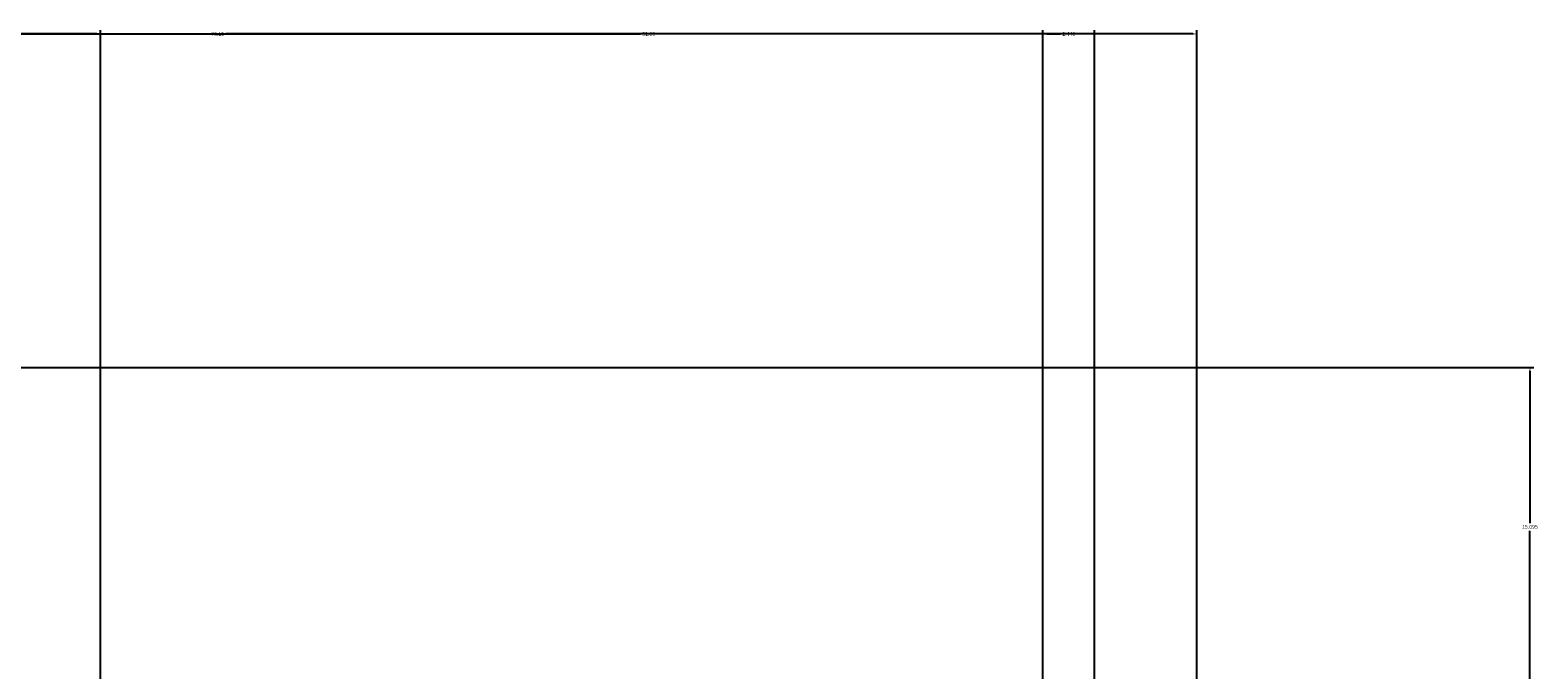
# Model space of a CAD drawing. Units: feet. Extents: x 2695 to 2912, y 795 to 1139.
# Tile 83 of 83: x 2840 to 2912, y 1109 to 1139. Entities that reach past the tile are written whole.
import ezdxf

# ---------------------------------------------------------------- set-up
doc = ezdxf.new("R2010")
doc.units = ezdxf.units.FT
doc.layers.add('A-ANNO-DIMS', color=2, linetype='Continuous', lineweight=18)
doc.styles.get("Standard").update_dxf_attribs({"font": 'arial.ttf'})
doc.dimstyles.get("Standard").update_dxf_attribs({"dimtxt": 0.18, "dimasz": 0.18, "dimexe": 0.18, "dimexo": 0.0625, "dimgap": 0.09, "dimtad": 0, "dimtih": 1, "dimtoh": 1, "dimdec": 1, "dimzin": 0, "dimdsep": 46, "dimlunit": 3, "dimtxsty": 'Standard', "dimcen": 0.09, "dimadec": 0, "dimazin": 0, "dimtfac": 1, "dimtdec": 1, "dimtofl": 0, "dimtmove": 0, "dimatfit": 3, "dimfxl": 1, "dimtolj": 1, "dimtzin": 0, "dimarcsym": 0})

# ---------------------------------------------------------------- blocks, each defined once
blk = doc.blocks.new('*D10')
at = {"layer": 'A-ANNO-DIMS', "color": 0, "lineweight": -2, "transparency": 16777216}
for p, q in [((2778.034, 1020.886), (2778.034, 1138.886)), ((2778.214, 1138.706), (2810.411, 1138.706)), ((2843.395, 1138.706), (2811.198, 1138.706)), ((2843.575, 1020.886), (2843.575, 1138.886))]:
    blk.add_line(p, q, dxfattribs=at)
at = {"layer": 'A-ANNO-DIMS', "color": 0, "transparency": 16777216}
for points in [[(2778.214, 1138.736), (2778.214, 1138.676), (2778.034, 1138.706)], [(2843.395, 1138.736), (2843.395, 1138.676), (2843.575, 1138.706)]]:
    blk.add_solid(points, dxfattribs=at)
at = {"layer": 'Defpoints', "color": 0, "transparency": 16777216}
for p in [(2843.575, 1138.706), (2778.034, 1020.824), (2843.575, 1020.824)]:
    blk.add_point(p, dxfattribs=at)
at = {"layer": 'A-ANNO-DIMS', "color": 0, "transparency": 16777216, "insert": (2810.805, 1138.706), "char_height": 0.18, "attachment_point": 5}
blk.add_mtext('\\A1;65.54', dxfattribs=at)
blk = doc.blocks.new('*D11')
at = {"layer": 'A-ANNO-DIMS', "color": 0, "lineweight": -2, "transparency": 16777216}
for p, q in [((2843.575, 1020.886), (2843.575, 1138.886)), ((2843.755, 1138.706), (2869.128, 1138.706)), ((2895.289, 1138.706), (2869.916, 1138.706)), ((2895.469, 1107.898), (2895.469, 1138.886))]:
    blk.add_line(p, q, dxfattribs=at)
at = {"layer": 'A-ANNO-DIMS', "color": 0, "transparency": 16777216}
for points in [[(2843.755, 1138.736), (2843.755, 1138.676), (2843.575, 1138.706)], [(2895.289, 1138.736), (2895.289, 1138.676), (2895.469, 1138.706)]]:
    blk.add_solid(points, dxfattribs=at)
at = {"layer": 'Defpoints', "color": 0, "transparency": 16777216}
for p in [(2895.469, 1138.706), (2895.469, 1107.835), (2843.575, 1020.824)]:
    blk.add_point(p, dxfattribs=at)
at = {"layer": 'A-ANNO-DIMS', "color": 0, "transparency": 16777216, "insert": (2869.522, 1138.706), "char_height": 0.18, "attachment_point": 5}
blk.add_mtext('\\A1;51.89', dxfattribs=at)
blk = doc.blocks.new('*D22')
at = {"layer": 'A-ANNO-DIMS', "color": 0, "lineweight": -2, "transparency": 16777216}
for p, q in [((2770.699, 1122.931), (2911.424, 1122.931)), ((2911.244, 1122.751), (2911.244, 1115.565)), ((2911.244, 1108.015), (2911.244, 1115.201)), ((2895.532, 1107.835), (2911.424, 1107.835))]:
    blk.add_line(p, q, dxfattribs=at)
at = {"layer": 'A-ANNO-DIMS', "color": 0, "transparency": 16777216}
for points in [[(2911.214, 1122.751), (2911.274, 1122.751), (2911.244, 1122.931)], [(2911.214, 1108.015), (2911.274, 1108.015), (2911.244, 1107.835)]]:
    blk.add_solid(points, dxfattribs=at)
at = {"layer": 'Defpoints', "color": 0, "transparency": 16777216}
for p in [(2770.636, 1122.931), (2911.244, 1122.931), (2895.469, 1107.835)]:
    blk.add_point(p, dxfattribs=at)
at = {"layer": 'A-ANNO-DIMS', "color": 0, "transparency": 16777216, "insert": (2911.244, 1115.383), "char_height": 0.18, "attachment_point": 5}
blk.add_mtext('\\A1;15.095', dxfattribs=at)
blk = doc.blocks.new('*D50')
at = {"layer": 'A-ANNO-DIMS', "color": 0, "lineweight": -2, "transparency": 16777216}
for p, q in [((2810.041, 972.03), (2810.041, 1138.886)), ((2810.221, 1138.706), (2848.721, 1138.706)), ((2888.008, 1138.706), (2849.508, 1138.706)), ((2888.188, 972.03), (2888.188, 1138.886))]:
    blk.add_line(p, q, dxfattribs=at)
at = {"layer": 'A-ANNO-DIMS', "color": 0, "transparency": 16777216}
for points in [[(2810.221, 1138.736), (2810.221, 1138.676), (2810.041, 1138.706)], [(2888.008, 1138.736), (2888.008, 1138.676), (2888.188, 1138.706)]]:
    blk.add_solid(points, dxfattribs=at)
at = {"layer": 'Defpoints', "color": 0, "transparency": 16777216}
for p in [(2888.188, 1138.706), (2810.041, 971.967), (2888.188, 971.967)]:
    blk.add_point(p, dxfattribs=at)
at = {"layer": 'A-ANNO-DIMS', "color": 0, "transparency": 16777216, "insert": (2849.114, 1138.706), "char_height": 0.18, "attachment_point": 5}
blk.add_mtext('\\A1;78.15', dxfattribs=at)
blk = doc.blocks.new('*D51')
at = {"layer": 'A-ANNO-DIMS', "color": 0, "lineweight": -2, "transparency": 16777216}
for p, q in [((2888.188, 972.03), (2888.188, 1138.886)), ((2888.368, 1138.706), (2889.017, 1138.706)), ((2890.456, 1138.706), (2889.808, 1138.706)), ((2890.636, 972.03), (2890.636, 1138.886))]:
    blk.add_line(p, q, dxfattribs=at)
at = {"layer": 'A-ANNO-DIMS', "color": 0, "transparency": 16777216}
for points in [[(2888.368, 1138.736), (2888.368, 1138.676), (2888.188, 1138.706)], [(2890.456, 1138.736), (2890.456, 1138.676), (2890.636, 1138.706)]]:
    blk.add_solid(points, dxfattribs=at)
at = {"layer": 'Defpoints', "color": 0, "transparency": 16777216}
for p in [(2890.636, 1138.706), (2888.188, 971.967), (2890.636, 971.967)]:
    blk.add_point(p, dxfattribs=at)
at = {"layer": 'A-ANNO-DIMS', "color": 0, "transparency": 16777216, "insert": (2889.412, 1138.706), "char_height": 0.18, "attachment_point": 5}
blk.add_mtext('\\A1;2.448', dxfattribs=at)

msp = doc.modelspace()

# ---------------------------------------------------------------- dimensions: what is measured, and where the dimension line sits
at = {"layer": 'A-ANNO-DIMS'}
for base, p1, p2, override, picture, middle in [((2843.575, 1138.7056), (2778.0341, 1020.8235), (2843.575, 1020.8235), {"dimdec": 2, "dimlfac": 1, "dimrnd": 0, "dimzin": 0, "dimdsep": 46, "dimlunit": 2}, '*D10', (2810.8045, 1138.7056)), ((2888.1882, 1138.7056), (2810.0407, 971.9673), (2888.1882, 971.9673), {"dimdec": 2, "dimlfac": 1, "dimrnd": 0, "dimzin": 0, "dimdsep": 46, "dimlunit": 2}, '*D50', (2849.1144, 1138.7056)), ((2895.4694, 1138.7056), (2843.575, 1020.8235), (2895.4694, 1107.8352), {"dimdec": 2, "dimlfac": 1, "dimrnd": 0, "dimzin": 0, "dimdsep": 46, "dimlunit": 2}, '*D11', (2869.5222, 1138.7056)), ((2890.6361, 1138.7056), (2888.1882, 971.9673), (2890.6361, 971.9673), {"dimdec": 3, "dimlfac": 1, "dimrnd": 0, "dimzin": 0, "dimdsep": 46, "dimlunit": 2}, '*D51', (2889.4121, 1138.7056))]:
    dim = msp.add_linear_dim(base=base, p1=p1, p2=p2, dimstyle='Standard', override=override, dxfattribs=at)
    dim.commit()
    dim.dimension.update_dxf_attribs({"geometry": picture, "text_midpoint": middle})
dim = msp.add_linear_dim(base=(2911.2444, 1122.9306), p1=(2895.4694, 1107.8352), p2=(2770.6361, 1122.9306), angle=90, dimstyle='Standard', override={"dimdec": 3, "dimlfac": 1, "dimrnd": 0, "dimzin": 0, "dimdsep": 46, "dimlunit": 2}, dxfattribs=at)
dim.commit()
dim.dimension.update_dxf_attribs({"geometry": '*D22', "text_midpoint": (2911.2444, 1115.3829)})

doc.saveas('drawing.dxf')
